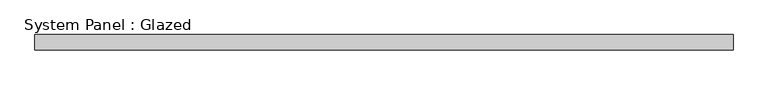
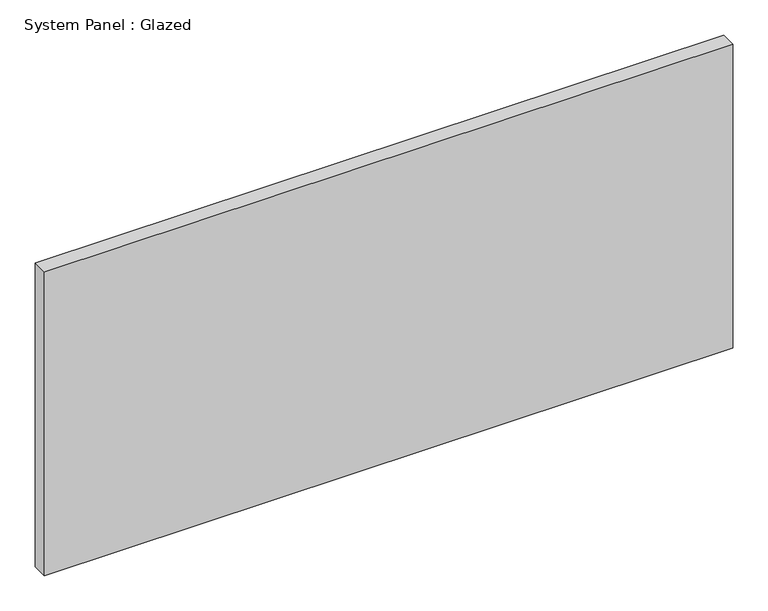
"""IFC4 building model written with IfcOpenShell, lengths in millimetres: plate geometry, System Panel : Glazed."""

from ifc_helpers import new_model, si_unit, origin, origin_with_axes, place, context, project, spatial, polyline, outline, extrude, source, transform, mapped, element, save


def system_panel_glazed_1d3ea9f9(model_context):
    return source(origin(), model_context, "Body", "SweptSolid", [
        extrude(outline(polyline([(562.5, 24.5), (-562.5, 24.5), (-562.5, 49.5), (562.5, 49.5), (562.5, 24.5)])), origin_with_axes(), (0.0, 0.0, 1.0), 525.0),
    ])


if __name__ == "__main__":
    model = new_model("IFC4")
    model_context = context("Model", 3, world=origin())
    ifc_project = project(units=[si_unit("LENGTHUNIT", "METRE", prefix="MILLI")], contexts=[model_context])
    site = spatial("IfcSite", under=ifc_project)
    building = spatial("IfcBuilding", under=site)
    placement = place(None, origin())
    system_panel_glazed_shape = system_panel_glazed_1d3ea9f9(model_context)
    element("IfcPlate", 1, ObjectType="System Panel : Glazed", at=placement, inside=building, context=model_context, shape_type="MappedRepresentation", body=[
        mapped(system_panel_glazed_shape, transform((0.0, 0.0, 0.0), x_axis=(1.0, 0.0, 0.0), y_axis=(0.0, 1.0, 0.0), z_axis=(0.0, 0.0, 1.0))),
    ])
    save(model, "model.ifc")

# Revit data of these elements
# Type "System Panel : Glazed"
#   Construction Type Id = "GSP4R"
#   Analytic Construction = "1/8 in Pilkington single glazing"
#   Visual Light Transmittance = 0.9
#   Solar Heat Gain Coefficient = 0.86
#   Heat Transfer Coefficient (U) = 6.7069 W/(m²·K)
#   Define Thermal Properties by = 1
# Element 1 (IfcPlate, "System Panel : Glazed")
#   Materials on its faces: "Glass"
# Materials
#   "Glass": class "Glass", colour RGB 245 245 243, transparency 1, Description = "Soda Lime Glass", Cost = 0
